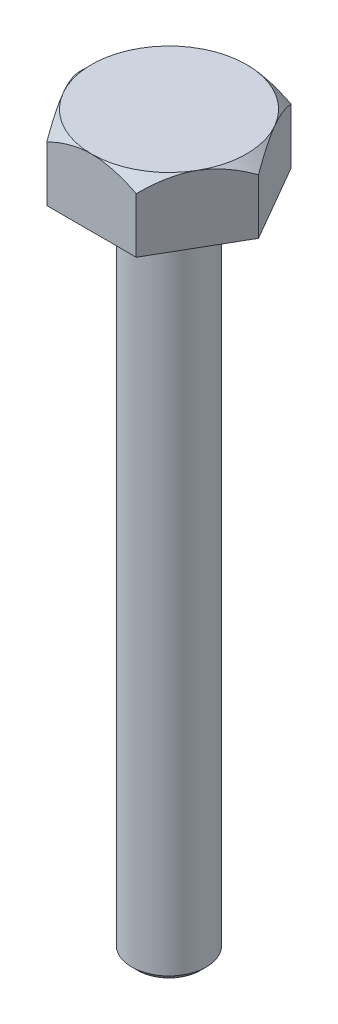
ISO-10303-21;
HEADER;
FILE_DESCRIPTION(('STEP AP214'),'2;1');
FILE_NAME('part.step','',(''),(''),'','','');
FILE_SCHEMA(('AUTOMOTIVE_DESIGN { 1 0 10303 214 1 1 1 1 }'));
ENDSEC;
DATA;
#1=APPLICATION_CONTEXT('core data for automotive mechanical design processes');
#2=APPLICATION_PROTOCOL_DEFINITION('international standard','automotive_design',2000,#1);
#3=PRODUCT_CONTEXT('',#1,'mechanical');
#4=PRODUCT('Part','Part','',(#3));
#5=PRODUCT_RELATED_PRODUCT_CATEGORY('part','',(#4));
#6=PRODUCT_DEFINITION_FORMATION('','',#4);
#7=PRODUCT_DEFINITION_CONTEXT('part definition',#1,'design');
#8=PRODUCT_DEFINITION('design','',#6,#7);
#9=PRODUCT_DEFINITION_SHAPE('','',#8);
#10=(LENGTH_UNIT() NAMED_UNIT(*) SI_UNIT(.MILLI.,.METRE.));
#11=(NAMED_UNIT(*) PLANE_ANGLE_UNIT() SI_UNIT($,.RADIAN.));
#12=(NAMED_UNIT(*) SI_UNIT($,.STERADIAN.) SOLID_ANGLE_UNIT());
#13=UNCERTAINTY_MEASURE_WITH_UNIT(LENGTH_MEASURE(1.E-05),#10,'distance_accuracy_value','');
#14=(GEOMETRIC_REPRESENTATION_CONTEXT(3) GLOBAL_UNCERTAINTY_ASSIGNED_CONTEXT((#13)) GLOBAL_UNIT_ASSIGNED_CONTEXT((#10,
#11,#12)) REPRESENTATION_CONTEXT('',''));
#15=CARTESIAN_POINT('',(0.,0.,0.));
#16=DIRECTION('',(0.,0.,1.));
#17=DIRECTION('',(1.,0.,0.));
#18=AXIS2_PLACEMENT_3D('',#15,#16,#17);
#19=CARTESIAN_POINT('',(-30.0222139978605,45.,52.));
#20=DIRECTION('',(0.,0.,-1.));
#21=DIRECTION('',(-1.,0.,0.));
#22=AXIS2_PLACEMENT_3D('',#19,#20,#21);
#23=PLANE('',#22);
#24=CARTESIAN_POINT('',(-104.974603519539,-20.1480575344053,52.));
#25=CARTESIAN_POINT('',(-103.444442169708,-18.7769494356472,52.));
#26=CARTESIAN_POINT('',(-101.911384838102,-17.4090635637915,52.));
#27=CARTESIAN_POINT('',(-98.8386625300546,-14.680700729552,52.));
#28=CARTESIAN_POINT('',(-97.2989974806682,-13.3202238493363,52.));
#29=CARTESIAN_POINT('',(-94.2117655194995,-10.6072235850642,52.));
#30=CARTESIAN_POINT('',(-92.664196154111,-9.25470299139133,52.));
#31=CARTESIAN_POINT('',(-89.5606976427889,-6.55929062983141,52.));
#32=CARTESIAN_POINT('',(-88.0047685189832,-5.2163988364791,52.));
#33=CARTESIAN_POINT('',(-84.8665982537161,-2.52727361111867,52.));
#34=CARTESIAN_POINT('',(-83.2842542569196,-1.18116012717798,52.));
#35=CARTESIAN_POINT('',(-80.1084838043138,1.49794750629656,52.));
#36=CARTESIAN_POINT('',(-78.5150573248629,2.83094162782893,52.));
#37=CARTESIAN_POINT('',(-75.3157667376626,5.48135702448698,52.));
#38=CARTESIAN_POINT('',(-73.7099048716653,6.79878100306021,52.));
#39=CARTESIAN_POINT('',(-70.4835124655795,9.4155570233478,52.));
#40=CARTESIAN_POINT('',(-68.8629819723785,10.7149091227943,52.));
#41=CARTESIAN_POINT('',(-65.7252946964395,13.1968820674329,52.));
#42=CARTESIAN_POINT('',(-64.2093494345498,14.3810328857299,52.));
#43=CARTESIAN_POINT('',(-61.1606138406127,16.7275072656802,52.));
#44=CARTESIAN_POINT('',(-59.6278234019294,17.8898306890322,52.));
#45=CARTESIAN_POINT('',(-56.5419574813941,20.1889777107931,52.));
#46=CARTESIAN_POINT('',(-54.9888717926023,21.3257876303724,52.));
#47=CARTESIAN_POINT('',(-51.8600616034661,23.5678926917397,52.));
#48=CARTESIAN_POINT('',(-50.2843374479378,24.6731883127718,52.));
#49=CARTESIAN_POINT('',(-47.9027588961038,26.3010577204605,52.));
#50=CARTESIAN_POINT('',(-47.1067786209454,26.8380990869268,52.));
#51=CARTESIAN_POINT('',(-45.5077429876137,27.9015346461807,52.));
#52=CARTESIAN_POINT('',(-44.7046877300736,28.4279289900598,52.));
#53=CARTESIAN_POINT('',(-43.09085839563,29.4689559851113,52.));
#54=CARTESIAN_POINT('',(-42.2800834844557,29.9835873441311,52.));
#55=CARTESIAN_POINT('',(-40.6503308676235,30.9996707599405,52.));
#56=CARTESIAN_POINT('',(-39.8313533365432,31.5011230964014,52.));
#57=CARTESIAN_POINT('',(-38.1852760607041,32.4888985857804,52.));
#58=CARTESIAN_POINT('',(-37.3581839506433,32.975234444567,52.));
#59=CARTESIAN_POINT('',(-35.6945351895526,33.9314936100802,52.));
#60=CARTESIAN_POINT('',(-34.8579784034972,34.4014166822659,52.));
#61=CARTESIAN_POINT('',(-33.1749408969925,35.3227686623054,52.));
#62=CARTESIAN_POINT('',(-32.3284621837012,35.7742012304012,52.));
#63=CARTESIAN_POINT('',(-30.6248353182834,36.6564043219331,52.));
#64=CARTESIAN_POINT('',(-29.7676877068093,37.0871758870515,52.));
#65=CARTESIAN_POINT('',(-28.1014002469777,37.8967384425179,52.));
#66=CARTESIAN_POINT('',(-27.2930086854749,38.2770672919812,52.));
#67=CARTESIAN_POINT('',(-25.6660607005647,39.0153364246869,52.));
#68=CARTESIAN_POINT('',(-24.8475044775925,39.3732771485594,52.));
#69=CARTESIAN_POINT('',(-23.1998803156875,40.0642892826952,52.));
#70=CARTESIAN_POINT('',(-22.3708117857534,40.3973592874115,52.));
#71=CARTESIAN_POINT('',(-20.702073505453,41.0358896387952,52.));
#72=CARTESIAN_POINT('',(-19.862403698907,41.3413498390793,52.));
#73=CARTESIAN_POINT('',(-18.1762063413501,41.9205092993988,52.));
#74=CARTESIAN_POINT('',(-17.3297241511565,42.1943402003845,52.));
#75=CARTESIAN_POINT('',(-15.626734785493,42.7087845664855,52.));
#76=CARTESIAN_POINT('',(-14.7702281113905,42.949399685228,52.));
#77=CARTESIAN_POINT('',(-13.0478359049288,43.3944593584753,52.));
#78=CARTESIAN_POINT('',(-12.1819504308002,43.5989041374158,52.));
#79=CARTESIAN_POINT('',(-10.4418517197723,43.9687867466574,52.));
#80=CARTESIAN_POINT('',(-9.56763847282889,44.134224529906,52.));
#81=CARTESIAN_POINT('',(-7.79708737906465,44.4260605485028,52.));
#82=CARTESIAN_POINT('',(-6.9006289245866,44.5517311226506,52.));
#83=CARTESIAN_POINT('',(-5.10250864919229,44.7578905629406,52.));
#84=CARTESIAN_POINT('',(-4.20084684342538,44.8383795605602,52.));
#85=CARTESIAN_POINT('',(-2.39467100795442,44.9526915724833,52.));
#86=CARTESIAN_POINT('',(-1.49015736317976,44.9865206354127,52.));
#87=CARTESIAN_POINT('',(0.319405672869893,45.006889864112,52.));
#88=CARTESIAN_POINT('',(1.22445506460228,44.9934299894499,52.));
#89=CARTESIAN_POINT('',(3.03386911749646,44.919427081205,52.));
#90=CARTESIAN_POINT('',(3.93823110670625,44.8588190475472,52.));
#91=CARTESIAN_POINT('',(5.74266334205835,44.6915772321508,52.));
#92=CARTESIAN_POINT('',(6.64273359815255,44.5849435571916,52.));
#93=CARTESIAN_POINT('',(8.4367191402026,44.3275220036307,52.));
#94=CARTESIAN_POINT('',(9.3306329712175,44.1767240310471,52.));
#95=CARTESIAN_POINT('',(11.1104092248204,43.8334830356432,52.));
#96=CARTESIAN_POINT('',(11.9962713736148,43.6410386021344,52.));
#97=CARTESIAN_POINT('',(13.9673809097387,43.1672161224463,52.));
#98=CARTESIAN_POINT('',(15.050162325768,42.8755698359679,52.));
#99=CARTESIAN_POINT('',(17.199882392269,42.2388692101925,52.));
#100=CARTESIAN_POINT('',(18.2668196987303,41.8938103681036,52.));
#101=CARTESIAN_POINT('',(20.3844311305142,41.1561144157292,52.));
#102=CARTESIAN_POINT('',(21.435099820739,40.7634617760078,52.));
#103=CARTESIAN_POINT('',(23.5197432427476,39.9363267728805,52.));
#104=CARTESIAN_POINT('',(24.5537182535443,39.5018451094386,52.));
#105=CARTESIAN_POINT('',(26.617528684912,38.5908799093831,52.));
#106=CARTESIAN_POINT('',(27.6471714147959,38.1139613893689,52.));
#107=CARTESIAN_POINT('',(29.6905952704967,37.127377922496,52.));
#108=CARTESIAN_POINT('',(30.7043763240441,36.6177128264905,52.));
#109=CARTESIAN_POINT('',(32.7167190987185,35.5699916340616,52.));
#110=CARTESIAN_POINT('',(33.7152855879172,35.0319446782918,52.));
#111=CARTESIAN_POINT('',(35.2027091269047,34.2062038320033,52.));
#112=CARTESIAN_POINT('',(35.6967798168579,33.927844828386,52.));
#113=CARTESIAN_POINT('',(36.6815952247146,33.3652920044684,52.));
#114=CARTESIAN_POINT('',(37.1723399145891,33.0810981350774,52.));
#115=CARTESIAN_POINT('',(38.4627450247686,32.3241817303639,52.));
#116=CARTESIAN_POINT('',(39.2597166191444,31.8468695967498,52.));
#117=CARTESIAN_POINT('',(40.8456504803188,30.8791046473685,52.));
#118=CARTESIAN_POINT('',(41.634612523387,30.3886514659184,52.));
#119=CARTESIAN_POINT('',(43.9904571033975,28.8995073949854,52.));
#120=CARTESIAN_POINT('',(45.5461685713643,27.883108504139,52.));
#121=CARTESIAN_POINT('',(48.6324575998831,25.8114617071009,52.));
#122=CARTESIAN_POINT('',(50.1630226887238,24.7561953178764,52.));
#123=CARTESIAN_POINT('',(53.201750110714,22.6140796743748,52.));
#124=CARTESIAN_POINT('',(54.7099133781582,21.5272317428642,52.));
#125=CARTESIAN_POINT('',(57.710912846122,19.3243364554514,52.));
#126=CARTESIAN_POINT('',(59.2036974407832,18.2082189541388,52.));
#127=CARTESIAN_POINT('',(62.1724441153612,15.9538389324413,52.));
#128=CARTESIAN_POINT('',(63.6484060467436,14.815576216767,52.));
#129=CARTESIAN_POINT('',(66.5853088929478,12.5206289542413,52.));
#130=CARTESIAN_POINT('',(68.0462535581434,11.3639492002705,52.));
#131=CARTESIAN_POINT('',(70.9553551542158,9.0346475086844,52.));
#132=CARTESIAN_POINT('',(72.4035121356618,7.86202563415925,52.));
#133=CARTESIAN_POINT('',(75.1757977039992,5.59532448057323,52.));
#134=CARTESIAN_POINT('',(76.5007688916879,4.50227464071074,52.));
#135=CARTESIAN_POINT('',(79.1422374587787,2.3059909642823,52.));
#136=CARTESIAN_POINT('',(80.4587348436884,1.20275713433677,52.));
#137=CARTESIAN_POINT('',(83.0842587401692,-1.01274333093366,52.));
#138=CARTESIAN_POINT('',(84.3932847278744,-2.12501058671541,52.));
#139=CARTESIAN_POINT('',(87.0045660739479,-4.35746560380634,52.));
#140=CARTESIAN_POINT('',(88.3068214204755,-5.47765337895888,52.));
#141=CARTESIAN_POINT('',(90.8973931655344,-7.71826962519173,52.));
#142=CARTESIAN_POINT('',(92.185746238517,-8.83865571159717,52.));
#143=CARTESIAN_POINT('',(94.7570301747009,-11.0856338234656,52.));
#144=CARTESIAN_POINT('',(96.0399610313417,-12.2122258564337,52.));
#145=CARTESIAN_POINT('',(98.6007446717763,-14.4708145356289,52.));
#146=CARTESIAN_POINT('',(99.8785981218244,-15.6028104267575,52.));
#147=CARTESIAN_POINT('',(102.42983830778,-17.8718111259995,52.));
#148=CARTESIAN_POINT('',(103.703225068163,-19.0088159065893,52.));
#149=CARTESIAN_POINT('',(104.974603519539,-20.1480575344052,52.));
#150=B_SPLINE_CURVE_WITH_KNOTS('',3,(#24,#25,#26,#27,#28,#29,#30,#31,#32,#33,#34,#35,#36,#37,
#38,#39,#40,#41,#42,#43,#44,#45,#46,#47,#48,#49,#50,#51,#52,#53,#54,#55,#56,#57,#58,#59,#60,#61,
#62,#63,#64,#65,#66,#67,#68,#69,#70,#71,#72,#73,#74,#75,#76,#77,#78,#79,#80,#81,#82,#83,#84,#85,
#86,#87,#88,#89,#90,#91,#92,#93,#94,#95,#96,#97,#98,#99,#100,#101,#102,#103,#104,#105,#106,#107,
#108,#109,#110,#111,#112,#113,#114,#115,#116,#117,#118,#119,#120,#121,#122,#123,#124,#125,#126,
#127,#128,#129,#130,#131,#132,#133,#134,#135,#136,#137,#138,#139,#140,#141,#142,#143,#144,#145,
#146,#147,#148,#149),.UNSPECIFIED.,.F.,.F.,(4,2,2,2,2,2,2,2,2,2,2,2,2,2,2,2,2,2,2,2,2,2,2,2,2,2,
2,2,2,2,2,2,2,2,2,2,2,2,2,2,2,2,2,2,2,2,2,2,2,2,2,2,2,2,2,2,2,2,2,2,2,2,4),(0.,6.16376855195753,
12.3276053234916,18.493488395418,24.6593551544522,30.8916696404896,37.1239974256607,
43.3552267046366,49.5864360728412,55.3571233374888,61.1278471536516,66.9015943485739,
72.6752536941409,75.5558064266588,78.4363182526549,81.3171449940328,84.1979105520807,
87.0761853944353,89.9545013508952,92.8322447563134,95.7098429194175,98.3897109444312,
101.069526209232,103.74949280703,106.429473612808,109.09786454091,111.766122576876,
114.434364055812,117.102608753327,119.817178750423,122.531740848134,125.245951018343,
127.960163509202,130.678124552666,133.396079290505,136.114655716595,138.833324243306,
142.19585187024,145.558663119932,148.922574594002,152.286429786384,155.689963480925,
159.093512678226,162.495972343473,164.197205953724,165.898453882901,168.685217983057,
171.472059712695,177.046194286842,182.623014702026,188.199601872464,193.791062080716,
199.382571620079,204.972649057908,210.562704379728,215.715585071901,220.868462414519,
226.021696724868,231.174940044188,236.297033600975,241.419133353498,246.540537187855,
251.661912915344),.UNSPECIFIED.);
#151=CARTESIAN_POINT('',(-30.0222139978605,36.9555720042789,52.));
#152=VERTEX_POINT('',#151);
#153=CARTESIAN_POINT('',(0.,45.,52.));
#154=VERTEX_POINT('',#153);
#155=EDGE_CURVE('E222',#152,#154,#150,.T.);
#156=ORIENTED_EDGE('',*,*,#155,.F.);
#157=DIRECTION('',(0.,-1.,0.));
#158=VECTOR('',#157,1.);
#159=CARTESIAN_POINT('',(-30.0222139978605,45.,52.));
#160=LINE('',#159,#158);
#161=CARTESIAN_POINT('',(-30.0222139978605,0.,52.));
#162=VERTEX_POINT('',#161);
#163=EDGE_CURVE('E221',#152,#162,#160,.T.);
#164=ORIENTED_EDGE('',*,*,#163,.T.);
#165=DIRECTION('',(1.,0.,0.));
#166=VECTOR('',#165,1.);
#167=CARTESIAN_POINT('',(-30.0222139978605,0.,52.));
#168=LINE('',#167,#166);
#169=CARTESIAN_POINT('',(30.0222139978605,0.,52.));
#170=VERTEX_POINT('',#169);
#171=EDGE_CURVE('E228',#162,#170,#168,.T.);
#172=ORIENTED_EDGE('',*,*,#171,.T.);
#173=DIRECTION('',(0.,-1.,0.));
#174=VECTOR('',#173,1.);
#175=CARTESIAN_POINT('',(30.0222139978605,45.,52.));
#176=LINE('',#175,#174);
#177=CARTESIAN_POINT('',(30.0222139978605,36.9555720042789,52.));
#178=VERTEX_POINT('',#177);
#179=EDGE_CURVE('E247',#178,#170,#176,.T.);
#180=ORIENTED_EDGE('',*,*,#179,.F.);
#181=EDGE_CURVE('E116',#154,#178,#150,.T.);
#182=ORIENTED_EDGE('',*,*,#181,.F.);
#183=EDGE_LOOP('',(#156,#164,#172,#180,#182));
#184=FACE_BOUND('',#183,.T.);
#185=ADVANCED_FACE('F45',(#184),#23,.F.);
#186=CARTESIAN_POINT('',(30.0222139978605,45.,52.));
#187=DIRECTION('',(-0.866025403784438,0.,-0.5));
#188=DIRECTION('',(-0.5,0.,0.866025403784439));
#189=AXIS2_PLACEMENT_3D('',#186,#187,#188);
#190=PLANE('',#189);
#191=CARTESIAN_POINT('',(30.0220985278067,36.955456533892,52.0002));
#192=CARTESIAN_POINT('',(30.280176534641,37.2135309803307,51.5531957798468));
#193=CARTESIAN_POINT('',(30.5392485388566,37.4676183415671,51.1044699057268));
#194=CARTESIAN_POINT('',(31.0594616022098,37.9672410148882,50.2034344492379));
#195=CARTESIAN_POINT('',(31.3206027677406,38.212775883668,49.7511246825909));
#196=CARTESIAN_POINT('',(32.107464297322,38.9358777611029,48.3882405348345));
#197=CARTESIAN_POINT('',(32.6363738806571,39.3996919544938,47.4721422638881));
#198=CARTESIAN_POINT('',(33.7060127767282,40.2877490866143,45.619473350141));
#199=CARTESIAN_POINT('',(34.2467924232445,40.7117502689875,44.6828155266756));
#200=CARTESIAN_POINT('',(35.3372385336309,41.5110185100584,42.7941074605706));
#201=CARTESIAN_POINT('',(35.8869036244094,41.8862930191751,41.8420595961952));
#202=CARTESIAN_POINT('',(36.9862330817044,42.5761964413529,39.9379651219031));
#203=CARTESIAN_POINT('',(37.5357617449106,42.8916856332666,38.9861535570145));
#204=CARTESIAN_POINT('',(38.6426137983935,43.462897464706,37.0690295639203));
#205=CARTESIAN_POINT('',(39.1999375700364,43.7186171691656,36.1037164751688));
#206=CARTESIAN_POINT('',(40.3198432183338,44.1637824175714,34.1639829926344));
#207=CARTESIAN_POINT('',(40.8824096700677,44.3533822155406,33.1895893155975));
#208=CARTESIAN_POINT('',(42.0123359693659,44.6621218387154,31.2324995564048));
#209=CARTESIAN_POINT('',(42.5796950878927,44.7812721913383,30.2498047369788));
#210=CARTESIAN_POINT('',(43.5552992194105,44.9223807751639,28.5600088131159));
#211=CARTESIAN_POINT('',(43.9629124532236,44.9623420710016,27.8540019823142));
#212=CARTESIAN_POINT('',(44.7786213959163,45.0038958786488,26.4411526493822));
#213=CARTESIAN_POINT('',(45.1867170795089,45.0054903193645,25.7343101910502));
#214=CARTESIAN_POINT('',(46.0026361970847,44.9702724935875,24.3210968245421));
#215=CARTESIAN_POINT('',(46.4104594797881,44.9334463746507,23.6147261783904));
#216=CARTESIAN_POINT('',(47.2248121036791,44.8219352098245,22.204226058534));
#217=CARTESIAN_POINT('',(47.6313414225626,44.747249514863,21.5000966234615));
#218=CARTESIAN_POINT('',(48.4427192287144,44.5610301112822,20.0947490390728));
#219=CARTESIAN_POINT('',(48.8475654352428,44.4494568192073,19.3935348401141));
#220=CARTESIAN_POINT('',(49.6544259013264,44.191061053402,17.9960115182386));
#221=CARTESIAN_POINT('',(50.0564401456341,44.044238390037,17.2997024217312));
#222=CARTESIAN_POINT('',(50.8569901438334,43.7172974585385,15.9131091508509));
#223=CARTESIAN_POINT('',(51.255526460246,43.537184683344,15.222824002163));
#224=CARTESIAN_POINT('',(52.0487663374305,43.1458008444998,13.8488922322897));
#225=CARTESIAN_POINT('',(52.4434695874179,42.9345272764499,13.165246149399));
#226=CARTESIAN_POINT('',(53.4596132305348,42.3503586126167,11.4052337317323));
#227=CARTESIAN_POINT('',(54.0779115662168,41.9554756092821,10.3343096000959));
#228=CARTESIAN_POINT('',(55.3033387530697,41.1021232134822,8.21180745149049));
#229=CARTESIAN_POINT('',(55.9104672666288,40.6436519026025,7.16023001928237));
#230=CARTESIAN_POINT('',(57.1117585467271,39.6733005330436,5.07953248746263));
#231=CARTESIAN_POINT('',(57.7059553438547,39.1615884431307,4.05035344514291));
#232=CARTESIAN_POINT('',(58.589037605449,38.3591005271834,2.5208101007988));
#233=CARTESIAN_POINT('',(58.8819529950742,38.0858616283834,2.01346576364905));
#234=CARTESIAN_POINT('',(59.4651752455835,37.5285665756802,1.00329519366237));
#235=CARTESIAN_POINT('',(59.7554822933588,37.2445112045562,0.500468637120165));
#236=CARTESIAN_POINT('',(60.0445434657749,36.955456533892,-0.000200000000003977));
#237=B_SPLINE_CURVE_WITH_KNOTS('',3,(#191,#192,#193,#194,#195,#196,#197,#198,#199,#200,#201,
#202,#203,#204,#205,#206,#207,#208,#209,#210,#211,#212,#213,#214,#215,#216,#217,#218,#219,#220,
#221,#222,#223,#224,#225,#226,#227,#228,#229,#230,#231,#232,#233,#234,#235,#236),.UNSPECIFIED.,
.F.,.F.,(4,2,2,2,2,2,2,2,2,2,2,2,2,2,2,2,2,2,2,2,2,2,4),(0.,1.73120255917828,3.46249471937643,
6.92674897903961,10.4108367985433,13.8943912642056,17.3232079778035,20.7521930329862,
24.1731240857042,27.5935438118124,30.041323321998,32.4889797690039,34.9375190179709,
37.3861002466024,39.8373175810715,42.2885481029052,44.7393745269956,47.1903980320222,
51.0825946301762,54.9749086787068,58.8552952790952,60.7944610079083,62.733486666627),.UNSPECIFIED.);
#238=CARTESIAN_POINT('',(45.0333209967908,45.,26.));
#239=VERTEX_POINT('',#238);
#240=EDGE_CURVE('E111',#178,#239,#237,.T.);
#241=ORIENTED_EDGE('',*,*,#240,.F.);
#242=ORIENTED_EDGE('',*,*,#179,.T.);
#243=DIRECTION('',(0.5,0.,-0.866025403784438));
#244=VECTOR('',#243,1.);
#245=CARTESIAN_POINT('',(30.0222139978605,0.,52.));
#246=LINE('',#245,#244);
#247=CARTESIAN_POINT('',(60.0444279957211,0.,0.));
#248=VERTEX_POINT('',#247);
#249=EDGE_CURVE('E257',#170,#248,#246,.T.);
#250=ORIENTED_EDGE('',*,*,#249,.T.);
#251=DIRECTION('',(0.,-1.,0.));
#252=VECTOR('',#251,1.);
#253=CARTESIAN_POINT('',(60.0444279957211,45.,0.));
#254=LINE('',#253,#252);
#255=CARTESIAN_POINT('',(60.0444279957211,36.9555720042789,0.));
#256=VERTEX_POINT('',#255);
#257=EDGE_CURVE('E141',#256,#248,#254,.T.);
#258=ORIENTED_EDGE('',*,*,#257,.F.);
#259=EDGE_CURVE('E124',#239,#256,#237,.T.);
#260=ORIENTED_EDGE('',*,*,#259,.F.);
#261=EDGE_LOOP('',(#241,#242,#250,#258,#260));
#262=FACE_BOUND('',#261,.T.);
#263=ADVANCED_FACE('F143',(#262),#190,.F.);
#264=CARTESIAN_POINT('',(60.0444279957211,45.,0.));
#265=DIRECTION('',(-0.866025403784439,0.,0.5));
#266=DIRECTION('',(0.5,0.,0.866025403784439));
#267=AXIS2_PLACEMENT_3D('',#264,#265,#266);
#268=PLANE('',#267);
#269=CARTESIAN_POINT('',(60.0445434657749,36.955456533892,0.000199999999997052));
#270=CARTESIAN_POINT('',(59.7864654589406,37.2135309803307,-0.446804220153167));
#271=CARTESIAN_POINT('',(59.527393454725,37.4676183415671,-0.895530094273238));
#272=CARTESIAN_POINT('',(59.0071803913718,37.9672410148882,-1.7965655507621));
#273=CARTESIAN_POINT('',(58.746039225841,38.212775883668,-2.24887531740914));
#274=CARTESIAN_POINT('',(57.9591776962596,38.9358777611029,-3.61175946516546));
#275=CARTESIAN_POINT('',(57.4302681129245,39.3996919544938,-4.52785773611194));
#276=CARTESIAN_POINT('',(56.3606292168534,40.2877490866143,-6.38052664985905));
#277=CARTESIAN_POINT('',(55.8198495703371,40.7117502689875,-7.31718447332443));
#278=CARTESIAN_POINT('',(54.7294034599507,41.5110185100584,-9.20589253942941));
#279=CARTESIAN_POINT('',(54.1797383691722,41.8862930191751,-10.1579404038048));
#280=CARTESIAN_POINT('',(53.0804089118772,42.5761964413529,-12.0620348780969));
#281=CARTESIAN_POINT('',(52.530880248671,42.8916856332666,-13.0138464429855));
#282=CARTESIAN_POINT('',(51.4240281951881,43.462897464706,-14.9309704360797));
#283=CARTESIAN_POINT('',(50.8667044235452,43.7186171691656,-15.8962835248312));
#284=CARTESIAN_POINT('',(49.7467987752478,44.1637824175714,-17.8360170073656));
#285=CARTESIAN_POINT('',(49.1842323235139,44.3533822155406,-18.8104106844025));
#286=CARTESIAN_POINT('',(48.0543060242157,44.6621218387154,-20.7675004435952));
#287=CARTESIAN_POINT('',(47.4869469056889,44.7812721913382,-21.7501952630212));
#288=CARTESIAN_POINT('',(46.5113427741711,44.9223807751638,-23.4399911868841));
#289=CARTESIAN_POINT('',(46.103729540358,44.9623420710016,-24.1459980176858));
#290=CARTESIAN_POINT('',(45.2880205976653,45.0038958786488,-25.5588473506178));
#291=CARTESIAN_POINT('',(44.8799249140727,45.0054903193645,-26.2656898089498));
#292=CARTESIAN_POINT('',(44.0640057964969,44.9702724935875,-27.6789031754579));
#293=CARTESIAN_POINT('',(43.6561825137935,44.9334463746507,-28.3852738216097));
#294=CARTESIAN_POINT('',(42.8418298899025,44.8219352098245,-29.795773941466));
#295=CARTESIAN_POINT('',(42.435300571019,44.747249514863,-30.4999033765385));
#296=CARTESIAN_POINT('',(41.6239227648672,44.5610301112822,-31.9052509609272));
#297=CARTESIAN_POINT('',(41.2190765583388,44.4494568192073,-32.606465159886));
#298=CARTESIAN_POINT('',(40.4122160922552,44.191061053402,-34.0039884817614));
#299=CARTESIAN_POINT('',(40.0102018479474,44.044238390037,-34.7002975782688));
#300=CARTESIAN_POINT('',(39.2096518497482,43.7172974585385,-36.0868908491491));
#301=CARTESIAN_POINT('',(38.8111155333356,43.537184683344,-36.777175997837));
#302=CARTESIAN_POINT('',(38.0178756561511,43.1458008444998,-38.1511077677104));
#303=CARTESIAN_POINT('',(37.6231724061637,42.9345272764499,-38.834753850601));
#304=CARTESIAN_POINT('',(36.6070287630468,42.3503586126167,-40.5947662682677));
#305=CARTESIAN_POINT('',(35.9887304273648,41.9554756092821,-41.6656903999042));
#306=CARTESIAN_POINT('',(34.7633032405119,41.1021232134821,-43.7881925485095));
#307=CARTESIAN_POINT('',(34.1561747269528,40.6436519026025,-44.8397699807176));
#308=CARTESIAN_POINT('',(32.9548834468545,39.6733005330436,-46.9204675125374));
#309=CARTESIAN_POINT('',(32.3606866497269,39.1615884431307,-47.9496465548571));
#310=CARTESIAN_POINT('',(31.4776043881327,38.3591005271834,-49.4791898992012));
#311=CARTESIAN_POINT('',(31.1846889985074,38.0858616283834,-49.9865342363509));
#312=CARTESIAN_POINT('',(30.6014667479982,37.5285665756802,-50.9967048063376));
#313=CARTESIAN_POINT('',(30.3111597002228,37.2445112045562,-51.4995313628798));
#314=CARTESIAN_POINT('',(30.0220985278067,36.955456533892,-52.0002));
#315=B_SPLINE_CURVE_WITH_KNOTS('',3,(#269,#270,#271,#272,#273,#274,#275,#276,#277,#278,#279,
#280,#281,#282,#283,#284,#285,#286,#287,#288,#289,#290,#291,#292,#293,#294,#295,#296,#297,#298,
#299,#300,#301,#302,#303,#304,#305,#306,#307,#308,#309,#310,#311,#312,#313,#314),.UNSPECIFIED.,
.F.,.F.,(4,2,2,2,2,2,2,2,2,2,2,2,2,2,2,2,2,2,2,2,2,2,4),(0.,1.73120255917828,3.46249471937644,
6.92674897903963,10.4108367985433,13.8943912642057,17.3232079778035,20.7521930329862,
24.1731240857042,27.5935438118124,30.0413233219981,32.4889797690039,34.937519017971,
37.3861002466024,39.8373175810715,42.2885481029052,44.7393745269956,47.1903980320223,
51.0825946301762,54.9749086787068,58.8552952790952,60.7944610079083,62.733486666627),.UNSPECIFIED.);
#316=CARTESIAN_POINT('',(45.0333209967908,45.,-26.));
#317=VERTEX_POINT('',#316);
#318=EDGE_CURVE('E129',#256,#317,#315,.T.);
#319=ORIENTED_EDGE('',*,*,#318,.F.);
#320=ORIENTED_EDGE('',*,*,#257,.T.);
#321=DIRECTION('',(-0.5,0.,-0.866025403784439));
#322=VECTOR('',#321,1.);
#323=CARTESIAN_POINT('',(60.0444279957211,0.,0.));
#324=LINE('',#323,#322);
#325=CARTESIAN_POINT('',(30.0222139978605,0.,-52.));
#326=VERTEX_POINT('',#325);
#327=EDGE_CURVE('E261',#248,#326,#324,.T.);
#328=ORIENTED_EDGE('',*,*,#327,.T.);
#329=DIRECTION('',(0.,-1.,0.));
#330=VECTOR('',#329,1.);
#331=CARTESIAN_POINT('',(30.0222139978605,45.,-52.));
#332=LINE('',#331,#330);
#333=CARTESIAN_POINT('',(30.0222139978605,36.9555720042789,-52.));
#334=VERTEX_POINT('',#333);
#335=EDGE_CURVE('E241',#334,#326,#332,.T.);
#336=ORIENTED_EDGE('',*,*,#335,.F.);
#337=EDGE_CURVE('E145',#317,#334,#315,.T.);
#338=ORIENTED_EDGE('',*,*,#337,.F.);
#339=EDGE_LOOP('',(#319,#320,#328,#336,#338));
#340=FACE_BOUND('',#339,.T.);
#341=ADVANCED_FACE('F206',(#340),#268,.F.);
#342=CARTESIAN_POINT('',(30.0222139978605,45.,-52.));
#343=DIRECTION('',(0.,0.,1.));
#344=DIRECTION('',(1.,0.,0.));
#345=AXIS2_PLACEMENT_3D('',#342,#343,#344);
#346=PLANE('',#345);
#347=CARTESIAN_POINT('',(104.974603519539,-20.1480575344053,-52.));
#348=CARTESIAN_POINT('',(103.444442169708,-18.7769494356472,-52.));
#349=CARTESIAN_POINT('',(101.911384838102,-17.4090635637915,-52.));
#350=CARTESIAN_POINT('',(98.8386625300547,-14.680700729552,-52.));
#351=CARTESIAN_POINT('',(97.2989974806683,-13.3202238493364,-52.));
#352=CARTESIAN_POINT('',(94.2117655194995,-10.6072235850642,-52.));
#353=CARTESIAN_POINT('',(92.6641961541111,-9.25470299139135,-52.));
#354=CARTESIAN_POINT('',(89.5606976427889,-6.55929062983143,-52.));
#355=CARTESIAN_POINT('',(88.0047685189833,-5.21639883647913,-52.));
#356=CARTESIAN_POINT('',(84.8665982537161,-2.52727361111871,-52.));
#357=CARTESIAN_POINT('',(83.2842542569196,-1.181160127178,-52.));
#358=CARTESIAN_POINT('',(80.1084838043138,1.49794750629655,-52.));
#359=CARTESIAN_POINT('',(78.5150573248629,2.83094162782891,-52.));
#360=CARTESIAN_POINT('',(75.3157667376626,5.48135702448695,-52.));
#361=CARTESIAN_POINT('',(73.7099048716654,6.79878100306017,-52.));
#362=CARTESIAN_POINT('',(70.4835124655795,9.41555702334776,-52.));
#363=CARTESIAN_POINT('',(68.8629819723785,10.7149091227943,-52.));
#364=CARTESIAN_POINT('',(65.7252946964395,13.1968820674329,-52.));
#365=CARTESIAN_POINT('',(64.2093494345498,14.3810328857299,-52.));
#366=CARTESIAN_POINT('',(61.1606138406127,16.7275072656802,-52.));
#367=CARTESIAN_POINT('',(59.6278234019294,17.8898306890322,-52.));
#368=CARTESIAN_POINT('',(56.5419574813941,20.1889777107931,-52.));
#369=CARTESIAN_POINT('',(54.9888717926024,21.3257876303723,-52.));
#370=CARTESIAN_POINT('',(51.8600616034662,23.5678926917397,-52.));
#371=CARTESIAN_POINT('',(50.2843374479378,24.6731883127717,-52.));
#372=CARTESIAN_POINT('',(47.9027588961038,26.3010577204604,-52.));
#373=CARTESIAN_POINT('',(47.1067786209455,26.8380990869267,-52.));
#374=CARTESIAN_POINT('',(45.5077429876137,27.9015346461807,-52.));
#375=CARTESIAN_POINT('',(44.7046877300736,28.4279289900597,-52.));
#376=CARTESIAN_POINT('',(43.09085839563,29.4689559851113,-52.));
#377=CARTESIAN_POINT('',(42.2800834844558,29.9835873441311,-52.));
#378=CARTESIAN_POINT('',(40.6503308676236,30.9996707599404,-52.));
#379=CARTESIAN_POINT('',(39.8313533365432,31.5011230964014,-52.));
#380=CARTESIAN_POINT('',(38.1852760607041,32.4888985857804,-52.));
#381=CARTESIAN_POINT('',(37.3581839506433,32.975234444567,-52.));
#382=CARTESIAN_POINT('',(35.6945351895526,33.9314936100802,-52.));
#383=CARTESIAN_POINT('',(34.8579784034973,34.4014166822659,-52.));
#384=CARTESIAN_POINT('',(33.1749408969925,35.3227686623054,-52.));
#385=CARTESIAN_POINT('',(32.3284621837013,35.7742012304011,-52.));
#386=CARTESIAN_POINT('',(30.6248353182834,36.6564043219331,-52.));
#387=CARTESIAN_POINT('',(29.7676877068093,37.0871758870515,-52.));
#388=CARTESIAN_POINT('',(28.1014002469778,37.8967384425179,-52.));
#389=CARTESIAN_POINT('',(27.2930086854749,38.2770672919812,-52.));
#390=CARTESIAN_POINT('',(25.6660607005647,39.0153364246868,-52.));
#391=CARTESIAN_POINT('',(24.8475044775926,39.3732771485593,-52.));
#392=CARTESIAN_POINT('',(23.1998803156876,40.0642892826952,-52.));
#393=CARTESIAN_POINT('',(22.3708117857535,40.3973592874115,-52.));
#394=CARTESIAN_POINT('',(20.7020735054531,41.0358896387952,-52.));
#395=CARTESIAN_POINT('',(19.8624036989071,41.3413498390792,-52.));
#396=CARTESIAN_POINT('',(18.1762063413502,41.9205092993988,-52.));
#397=CARTESIAN_POINT('',(17.3297241511565,42.1943402003845,-52.));
#398=CARTESIAN_POINT('',(15.626734785493,42.7087845664855,-52.));
#399=CARTESIAN_POINT('',(14.7702281113905,42.949399685228,-52.));
#400=CARTESIAN_POINT('',(13.0478359049289,43.3944593584753,-52.));
#401=CARTESIAN_POINT('',(12.1819504308002,43.5989041374157,-52.));
#402=CARTESIAN_POINT('',(10.4418517197723,43.9687867466574,-52.));
#403=CARTESIAN_POINT('',(9.56763847282894,44.1342245299059,-52.));
#404=CARTESIAN_POINT('',(7.7970873790647,44.4260605485027,-52.));
#405=CARTESIAN_POINT('',(6.90062892458666,44.5517311226506,-52.));
#406=CARTESIAN_POINT('',(5.10250864919234,44.7578905629406,-52.));
#407=CARTESIAN_POINT('',(4.20084684342543,44.8383795605602,-52.));
#408=CARTESIAN_POINT('',(2.39467100795447,44.9526915724833,-52.));
#409=CARTESIAN_POINT('',(1.49015736317981,44.9865206354127,-52.));
#410=CARTESIAN_POINT('',(-0.319405672869844,45.006889864112,-52.));
#411=CARTESIAN_POINT('',(-1.22445506460223,44.9934299894499,-52.));
#412=CARTESIAN_POINT('',(-3.0338691174964,44.919427081205,-52.));
#413=CARTESIAN_POINT('',(-3.9382311067062,44.8588190475472,-52.));
#414=CARTESIAN_POINT('',(-5.74266334205829,44.6915772321508,-52.));
#415=CARTESIAN_POINT('',(-6.64273359815248,44.5849435571916,-52.));
#416=CARTESIAN_POINT('',(-8.43671914020252,44.3275220036307,-52.));
#417=CARTESIAN_POINT('',(-9.33063297121742,44.1767240310471,-52.));
#418=CARTESIAN_POINT('',(-11.1104092248203,43.8334830356432,-52.));
#419=CARTESIAN_POINT('',(-11.9962713736147,43.6410386021344,-52.));
#420=CARTESIAN_POINT('',(-13.9673809097387,43.1672161224463,-52.));
#421=CARTESIAN_POINT('',(-15.050162325768,42.8755698359679,-52.));
#422=CARTESIAN_POINT('',(-17.199882392269,42.2388692101925,-52.));
#423=CARTESIAN_POINT('',(-18.2668196987302,41.8938103681037,-52.));
#424=CARTESIAN_POINT('',(-20.3844311305141,41.1561144157292,-52.));
#425=CARTESIAN_POINT('',(-21.435099820739,40.7634617760079,-52.));
#426=CARTESIAN_POINT('',(-23.5197432427475,39.9363267728805,-52.));
#427=CARTESIAN_POINT('',(-24.5537182535442,39.5018451094386,-52.));
#428=CARTESIAN_POINT('',(-26.6175286849119,38.5908799093831,-52.));
#429=CARTESIAN_POINT('',(-27.6471714147958,38.1139613893689,-52.));
#430=CARTESIAN_POINT('',(-29.6905952704966,37.1273779224961,-52.));
#431=CARTESIAN_POINT('',(-30.704376324044,36.6177128264906,-52.));
#432=CARTESIAN_POINT('',(-32.7167190987184,35.5699916340616,-52.));
#433=CARTESIAN_POINT('',(-33.7152855879171,35.0319446782919,-52.));
#434=CARTESIAN_POINT('',(-35.2027091269046,34.2062038320034,-52.));
#435=CARTESIAN_POINT('',(-35.6967798168578,33.927844828386,-52.));
#436=CARTESIAN_POINT('',(-36.6815952247145,33.3652920044684,-52.));
#437=CARTESIAN_POINT('',(-37.172339914589,33.0810981350775,-52.));
#438=CARTESIAN_POINT('',(-38.4627450247685,32.324181730364,-52.));
#439=CARTESIAN_POINT('',(-39.2597166191443,31.8468695967499,-52.));
#440=CARTESIAN_POINT('',(-40.8456504803187,30.8791046473686,-52.));
#441=CARTESIAN_POINT('',(-41.6346125233869,30.3886514659184,-52.));
#442=CARTESIAN_POINT('',(-43.9904571033974,28.8995073949854,-52.));
#443=CARTESIAN_POINT('',(-45.5461685713642,27.8831085041391,-52.));
#444=CARTESIAN_POINT('',(-48.632457599883,25.811461707101,-52.));
#445=CARTESIAN_POINT('',(-50.1630226887237,24.7561953178765,-52.));
#446=CARTESIAN_POINT('',(-53.2017501107139,22.6140796743748,-52.));
#447=CARTESIAN_POINT('',(-54.7099133781582,21.5272317428642,-52.));
#448=CARTESIAN_POINT('',(-57.7109128461219,19.3243364554514,-52.));
#449=CARTESIAN_POINT('',(-59.2036974407832,18.2082189541388,-52.));
#450=CARTESIAN_POINT('',(-62.1724441153611,15.9538389324413,-52.));
#451=CARTESIAN_POINT('',(-63.6484060467436,14.815576216767,-52.));
#452=CARTESIAN_POINT('',(-66.5853088929477,12.5206289542414,-52.));
#453=CARTESIAN_POINT('',(-68.0462535581434,11.3639492002705,-52.));
#454=CARTESIAN_POINT('',(-70.9553551542158,9.03464750868444,-52.));
#455=CARTESIAN_POINT('',(-72.4035121356618,7.86202563415928,-52.));
#456=CARTESIAN_POINT('',(-75.1757977039992,5.59532448057327,-52.));
#457=CARTESIAN_POINT('',(-76.5007688916879,4.50227464071078,-52.));
#458=CARTESIAN_POINT('',(-79.1422374587786,2.30599096428233,-52.));
#459=CARTESIAN_POINT('',(-80.4587348436883,1.20275713433678,-52.));
#460=CARTESIAN_POINT('',(-83.0842587401691,-1.01274333093365,-52.));
#461=CARTESIAN_POINT('',(-84.3932847278744,-2.12501058671539,-52.));
#462=CARTESIAN_POINT('',(-87.0045660739478,-4.35746560380631,-52.));
#463=CARTESIAN_POINT('',(-88.3068214204755,-5.47765337895886,-52.));
#464=CARTESIAN_POINT('',(-90.8973931655344,-7.71826962519172,-52.));
#465=CARTESIAN_POINT('',(-92.185746238517,-8.83865571159716,-52.));
#466=CARTESIAN_POINT('',(-94.7570301747009,-11.0856338234656,-52.));
#467=CARTESIAN_POINT('',(-96.0399610313417,-12.2122258564337,-52.));
#468=CARTESIAN_POINT('',(-98.6007446717763,-14.4708145356289,-52.));
#469=CARTESIAN_POINT('',(-99.8785981218244,-15.6028104267576,-52.));
#470=CARTESIAN_POINT('',(-102.42983830778,-17.8718111259996,-52.));
#471=CARTESIAN_POINT('',(-103.703225068163,-19.0088159065893,-52.));
#472=CARTESIAN_POINT('',(-104.974603519539,-20.1480575344053,-52.));
#473=B_SPLINE_CURVE_WITH_KNOTS('',3,(#347,#348,#349,#350,#351,#352,#353,#354,#355,#356,#357,
#358,#359,#360,#361,#362,#363,#364,#365,#366,#367,#368,#369,#370,#371,#372,#373,#374,#375,#376,
#377,#378,#379,#380,#381,#382,#383,#384,#385,#386,#387,#388,#389,#390,#391,#392,#393,#394,#395,
#396,#397,#398,#399,#400,#401,#402,#403,#404,#405,#406,#407,#408,#409,#410,#411,#412,#413,#414,
#415,#416,#417,#418,#419,#420,#421,#422,#423,#424,#425,#426,#427,#428,#429,#430,#431,#432,#433,
#434,#435,#436,#437,#438,#439,#440,#441,#442,#443,#444,#445,#446,#447,#448,#449,#450,#451,#452,
#453,#454,#455,#456,#457,#458,#459,#460,#461,#462,#463,#464,#465,#466,#467,#468,#469,#470,#471,
#472),.UNSPECIFIED.,.F.,.F.,(4,2,2,2,2,2,2,2,2,2,2,2,2,2,2,2,2,2,2,2,2,2,2,2,2,2,2,2,2,2,2,2,2,
2,2,2,2,2,2,2,2,2,2,2,2,2,2,2,2,2,2,2,2,2,2,2,2,2,2,2,2,2,4),(0.,6.16376855195752,
12.3276053234915,18.493488395418,24.6593551544522,30.8916696404896,37.1239974256607,
43.3552267046366,49.5864360728412,55.3571233374888,61.1278471536517,66.9015943485739,
72.6752536941409,75.5558064266588,78.4363182526549,81.3171449940328,84.1979105520807,
87.0761853944353,89.9545013508952,92.8322447563134,95.7098429194175,98.3897109444312,
101.069526209232,103.74949280703,106.429473612808,109.09786454091,111.766122576876,
114.434364055812,117.102608753327,119.817178750423,122.531740848134,125.245951018343,
127.960163509202,130.678124552666,133.396079290505,136.114655716595,138.833324243306,
142.19585187024,145.558663119932,148.922574594002,152.286429786384,155.689963480925,
159.093512678226,162.495972343472,164.197205953724,165.898453882901,168.685217983057,
171.472059712694,177.046194286841,182.623014702026,188.199601872464,193.791062080715,
199.382571620079,204.972649057908,210.562704379728,215.715585071901,220.868462414519,
226.021696724868,231.174940044188,236.297033600975,241.419133353498,246.540537187855,
251.661912915344),.UNSPECIFIED.);
#474=CARTESIAN_POINT('',(0.,45.,-52.));
#475=VERTEX_POINT('',#474);
#476=EDGE_CURVE('E199',#334,#475,#473,.T.);
#477=ORIENTED_EDGE('',*,*,#476,.F.);
#478=ORIENTED_EDGE('',*,*,#335,.T.);
#479=DIRECTION('',(-1.,0.,0.));
#480=VECTOR('',#479,1.);
#481=CARTESIAN_POINT('',(30.0222139978605,0.,-52.));
#482=LINE('',#481,#480);
#483=CARTESIAN_POINT('',(-30.0222139978606,0.,-52.));
#484=VERTEX_POINT('',#483);
#485=EDGE_CURVE('E266',#326,#484,#482,.T.);
#486=ORIENTED_EDGE('',*,*,#485,.T.);
#487=DIRECTION('',(0.,-1.,0.));
#488=VECTOR('',#487,1.);
#489=CARTESIAN_POINT('',(-30.0222139978606,45.,-52.));
#490=LINE('',#489,#488);
#491=CARTESIAN_POINT('',(-30.0222139978606,36.9555720042789,-52.));
#492=VERTEX_POINT('',#491);
#493=EDGE_CURVE('E237',#492,#484,#490,.T.);
#494=ORIENTED_EDGE('',*,*,#493,.F.);
#495=EDGE_CURVE('E191',#475,#492,#473,.T.);
#496=ORIENTED_EDGE('',*,*,#495,.F.);
#497=EDGE_LOOP('',(#477,#478,#486,#494,#496));
#498=FACE_BOUND('',#497,.T.);
#499=ADVANCED_FACE('F205',(#498),#346,.F.);
#500=CARTESIAN_POINT('',(-30.0222139978606,45.,-52.));
#501=DIRECTION('',(0.866025403784439,0.,0.5));
#502=DIRECTION('',(0.5,0.,-0.866025403784439));
#503=AXIS2_PLACEMENT_3D('',#500,#501,#502);
#504=PLANE('',#503);
#505=CARTESIAN_POINT('',(-30.0220985278067,36.955456533892,-52.0002));
#506=CARTESIAN_POINT('',(-30.280176534641,37.2135309803307,-51.5531957798468));
#507=CARTESIAN_POINT('',(-30.5392485388566,37.4676183415671,-51.1044699057267));
#508=CARTESIAN_POINT('',(-31.0594616022099,37.9672410148882,-50.2034344492379));
#509=CARTESIAN_POINT('',(-31.3206027677406,38.212775883668,-49.7511246825908));
#510=CARTESIAN_POINT('',(-32.107464297322,38.9358777611029,-48.3882405348345));
#511=CARTESIAN_POINT('',(-32.6363738806571,39.3996919544938,-47.472142263888));
#512=CARTESIAN_POINT('',(-33.7060127767283,40.2877490866143,-45.6194733501409));
#513=CARTESIAN_POINT('',(-34.2467924232446,40.7117502689875,-44.6828155266755));
#514=CARTESIAN_POINT('',(-35.3372385336309,41.5110185100584,-42.7941074605706));
#515=CARTESIAN_POINT('',(-35.8869036244094,41.8862930191751,-41.8420595961952));
#516=CARTESIAN_POINT('',(-36.9862330817045,42.5761964413529,-39.937965121903));
#517=CARTESIAN_POINT('',(-37.5357617449107,42.8916856332666,-38.9861535570145));
#518=CARTESIAN_POINT('',(-38.6426137983935,43.462897464706,-37.0690295639203));
#519=CARTESIAN_POINT('',(-39.1999375700364,43.7186171691656,-36.1037164751688));
#520=CARTESIAN_POINT('',(-40.3198432183338,44.1637824175714,-34.1639829926344));
#521=CARTESIAN_POINT('',(-40.8824096700677,44.3533822155406,-33.1895893155975));
#522=CARTESIAN_POINT('',(-42.0123359693659,44.6621218387154,-31.2324995564048));
#523=CARTESIAN_POINT('',(-42.5796950878928,44.7812721913383,-30.2498047369788));
#524=CARTESIAN_POINT('',(-43.5552992194106,44.9223807751639,-28.5600088131159));
#525=CARTESIAN_POINT('',(-43.9629124532236,44.9623420710016,-27.8540019823141));
#526=CARTESIAN_POINT('',(-44.7786213959163,45.0038958786488,-26.4411526493822));
#527=CARTESIAN_POINT('',(-45.1867170795089,45.0054903193645,-25.7343101910502));
#528=CARTESIAN_POINT('',(-46.0026361970848,44.9702724935875,-24.3210968245421));
#529=CARTESIAN_POINT('',(-46.4104594797881,44.9334463746507,-23.6147261783903));
#530=CARTESIAN_POINT('',(-47.2248121036792,44.8219352098245,-22.204226058534));
#531=CARTESIAN_POINT('',(-47.6313414225626,44.747249514863,-21.5000966234615));
#532=CARTESIAN_POINT('',(-48.4427192287144,44.5610301112822,-20.0947490390728));
#533=CARTESIAN_POINT('',(-48.8475654352428,44.4494568192073,-19.393534840114));
#534=CARTESIAN_POINT('',(-49.6544259013264,44.191061053402,-17.9960115182386));
#535=CARTESIAN_POINT('',(-50.0564401456342,44.044238390037,-17.2997024217312));
#536=CARTESIAN_POINT('',(-50.8569901438334,43.7172974585385,-15.9131091508509));
#537=CARTESIAN_POINT('',(-51.255526460246,43.537184683344,-15.222824002163));
#538=CARTESIAN_POINT('',(-52.0487663374305,43.1458008444998,-13.8488922322897));
#539=CARTESIAN_POINT('',(-52.4434695874179,42.9345272764499,-13.165246149399));
#540=CARTESIAN_POINT('',(-53.4596132305348,42.3503586126167,-11.4052337317323));
#541=CARTESIAN_POINT('',(-54.0779115662168,41.9554756092821,-10.3343096000959));
#542=CARTESIAN_POINT('',(-55.3033387530697,41.1021232134821,-8.21180745149049));
#543=CARTESIAN_POINT('',(-55.9104672666288,40.6436519026025,-7.16023001928236));
#544=CARTESIAN_POINT('',(-57.1117585467271,39.6733005330436,-5.07953248746264));
#545=CARTESIAN_POINT('',(-57.7059553438547,39.1615884431308,-4.05035344514292));
#546=CARTESIAN_POINT('',(-58.589037605449,38.3591005271834,-2.52081010079882));
#547=CARTESIAN_POINT('',(-58.8819529950742,38.0858616283834,-2.01346576364906));
#548=CARTESIAN_POINT('',(-59.4651752455834,37.5285665756802,-1.00329519366239));
#549=CARTESIAN_POINT('',(-59.7554822933588,37.2445112045562,-0.500468637120186));
#550=CARTESIAN_POINT('',(-60.0445434657749,36.955456533892,0.000199999999983028));
#551=B_SPLINE_CURVE_WITH_KNOTS('',3,(#505,#506,#507,#508,#509,#510,#511,#512,#513,#514,#515,
#516,#517,#518,#519,#520,#521,#522,#523,#524,#525,#526,#527,#528,#529,#530,#531,#532,#533,#534,
#535,#536,#537,#538,#539,#540,#541,#542,#543,#544,#545,#546,#547,#548,#549,#550),.UNSPECIFIED.,
.F.,.F.,(4,2,2,2,2,2,2,2,2,2,2,2,2,2,2,2,2,2,2,2,2,2,4),(0.,1.73120255917829,3.46249471937644,
6.92674897903963,10.4108367985433,13.8943912642057,17.3232079778035,20.7521930329862,
24.1731240857042,27.5935438118125,30.0413233219981,32.4889797690039,34.937519017971,
37.3861002466024,39.8373175810715,42.2885481029052,44.7393745269956,47.1903980320223,
51.0825946301762,54.9749086787068,58.8552952790952,60.7944610079083,62.733486666627),.UNSPECIFIED.);
#552=CARTESIAN_POINT('',(-45.0333209967908,45.,-26.));
#553=VERTEX_POINT('',#552);
#554=EDGE_CURVE('E203',#492,#553,#551,.T.);
#555=ORIENTED_EDGE('',*,*,#554,.F.);
#556=ORIENTED_EDGE('',*,*,#493,.T.);
#557=DIRECTION('',(-0.5,0.,0.866025403784439));
#558=VECTOR('',#557,1.);
#559=CARTESIAN_POINT('',(-30.0222139978606,0.,-52.));
#560=LINE('',#559,#558);
#561=CARTESIAN_POINT('',(-60.0444279957211,0.,0.));
#562=VERTEX_POINT('',#561);
#563=EDGE_CURVE('E236',#484,#562,#560,.T.);
#564=ORIENTED_EDGE('',*,*,#563,.T.);
#565=DIRECTION('',(0.,-1.,0.));
#566=VECTOR('',#565,1.);
#567=CARTESIAN_POINT('',(-60.0444279957211,45.,0.));
#568=LINE('',#567,#566);
#569=CARTESIAN_POINT('',(-60.0444279957211,36.9555720042789,0.));
#570=VERTEX_POINT('',#569);
#571=EDGE_CURVE('E231',#570,#562,#568,.T.);
#572=ORIENTED_EDGE('',*,*,#571,.F.);
#573=EDGE_CURVE('E186',#553,#570,#551,.T.);
#574=ORIENTED_EDGE('',*,*,#573,.F.);
#575=EDGE_LOOP('',(#555,#556,#564,#572,#574));
#576=FACE_BOUND('',#575,.T.);
#577=ADVANCED_FACE('F202',(#576),#504,.F.);
#578=CARTESIAN_POINT('',(-60.0444279957211,45.,0.));
#579=DIRECTION('',(0.866025403784439,0.,-0.5));
#580=DIRECTION('',(-0.5,0.,-0.866025403784439));
#581=AXIS2_PLACEMENT_3D('',#578,#579,#580);
#582=PLANE('',#581);
#583=CARTESIAN_POINT('',(-60.0445434657749,36.955456533892,-0.000200000000013965));
#584=CARTESIAN_POINT('',(-59.7864654589406,37.2135309803307,0.446804220153151));
#585=CARTESIAN_POINT('',(-59.527393454725,37.4676183415671,0.895530094273222));
#586=CARTESIAN_POINT('',(-59.0071803913718,37.9672410148882,1.79656555076208));
#587=CARTESIAN_POINT('',(-58.746039225841,38.212775883668,2.24887531740912));
#588=CARTESIAN_POINT('',(-57.9591776962596,38.9358777611029,3.61175946516544));
#589=CARTESIAN_POINT('',(-57.4302681129245,39.3996919544938,4.52785773611192));
#590=CARTESIAN_POINT('',(-56.3606292168534,40.2877490866143,6.38052664985903));
#591=CARTESIAN_POINT('',(-55.8198495703371,40.7117502689875,7.31718447332441));
#592=CARTESIAN_POINT('',(-54.7294034599507,41.5110185100585,9.20589253942938));
#593=CARTESIAN_POINT('',(-54.1797383691722,41.8862930191751,10.1579404038047));
#594=CARTESIAN_POINT('',(-53.0804089118772,42.5761964413529,12.0620348780969));
#595=CARTESIAN_POINT('',(-52.530880248671,42.8916856332666,13.0138464429854));
#596=CARTESIAN_POINT('',(-51.4240281951881,43.462897464706,14.9309704360797));
#597=CARTESIAN_POINT('',(-50.8667044235452,43.7186171691656,15.8962835248312));
#598=CARTESIAN_POINT('',(-49.7467987752478,44.1637824175714,17.8360170073656));
#599=CARTESIAN_POINT('',(-49.1842323235139,44.3533822155406,18.8104106844025));
#600=CARTESIAN_POINT('',(-48.0543060242157,44.6621218387154,20.7675004435952));
#601=CARTESIAN_POINT('',(-47.4869469056889,44.7812721913383,21.7501952630212));
#602=CARTESIAN_POINT('',(-46.5113427741711,44.9223807751639,23.4399911868841));
#603=CARTESIAN_POINT('',(-46.103729540358,44.9623420710016,24.1459980176858));
#604=CARTESIAN_POINT('',(-45.2880205976653,45.0038958786488,25.5588473506178));
#605=CARTESIAN_POINT('',(-44.8799249140727,45.0054903193645,26.2656898089498));
#606=CARTESIAN_POINT('',(-44.0640057964969,44.9702724935875,27.6789031754579));
#607=CARTESIAN_POINT('',(-43.6561825137935,44.9334463746507,28.3852738216096));
#608=CARTESIAN_POINT('',(-42.8418298899025,44.8219352098245,29.7957739414659));
#609=CARTESIAN_POINT('',(-42.435300571019,44.7472495148631,30.4999033765385));
#610=CARTESIAN_POINT('',(-41.6239227648672,44.5610301112823,31.9052509609272));
#611=CARTESIAN_POINT('',(-41.2190765583388,44.4494568192073,32.6064651598859));
#612=CARTESIAN_POINT('',(-40.4122160922552,44.191061053402,34.0039884817614));
#613=CARTESIAN_POINT('',(-40.0102018479474,44.044238390037,34.7002975782688));
#614=CARTESIAN_POINT('',(-39.2096518497482,43.7172974585385,36.0868908491491));
#615=CARTESIAN_POINT('',(-38.8111155333356,43.537184683344,36.777175997837));
#616=CARTESIAN_POINT('',(-38.0178756561511,43.1458008444998,38.1511077677103));
#617=CARTESIAN_POINT('',(-37.6231724061637,42.9345272764499,38.834753850601));
#618=CARTESIAN_POINT('',(-36.6070287630468,42.3503586126167,40.5947662682677));
#619=CARTESIAN_POINT('',(-35.9887304273648,41.9554756092821,41.6656903999041));
#620=CARTESIAN_POINT('',(-34.7633032405119,41.1021232134822,43.7881925485095));
#621=CARTESIAN_POINT('',(-34.1561747269528,40.6436519026025,44.8397699807176));
#622=CARTESIAN_POINT('',(-32.9548834468545,39.6733005330436,46.9204675125373));
#623=CARTESIAN_POINT('',(-32.3606866497269,39.1615884431308,47.9496465548571));
#624=CARTESIAN_POINT('',(-31.4776043881327,38.3591005271835,49.4791898992012));
#625=CARTESIAN_POINT('',(-31.1846889985074,38.0858616283834,49.9865342363509));
#626=CARTESIAN_POINT('',(-30.6014667479982,37.5285665756802,50.9967048063376));
#627=CARTESIAN_POINT('',(-30.3111597002228,37.2445112045562,51.4995313628798));
#628=CARTESIAN_POINT('',(-30.0220985278067,36.955456533892,52.0002));
#629=B_SPLINE_CURVE_WITH_KNOTS('',3,(#583,#584,#585,#586,#587,#588,#589,#590,#591,#592,#593,
#594,#595,#596,#597,#598,#599,#600,#601,#602,#603,#604,#605,#606,#607,#608,#609,#610,#611,#612,
#613,#614,#615,#616,#617,#618,#619,#620,#621,#622,#623,#624,#625,#626,#627,#628),.UNSPECIFIED.,
.F.,.F.,(4,2,2,2,2,2,2,2,2,2,2,2,2,2,2,2,2,2,2,2,2,2,4),(0.,1.73120255917828,3.46249471937644,
6.92674897903963,10.4108367985433,13.8943912642057,17.3232079778035,20.7521930329862,
24.1731240857042,27.5935438118124,30.0413233219981,32.4889797690039,34.937519017971,
37.3861002466024,39.8373175810715,42.2885481029052,44.7393745269956,47.1903980320222,
51.0825946301762,54.9749086787068,58.8552952790952,60.7944610079083,62.733486666627),.UNSPECIFIED.);
#630=CARTESIAN_POINT('',(-45.0333209967908,45.,26.));
#631=VERTEX_POINT('',#630);
#632=EDGE_CURVE('E287',#570,#631,#629,.T.);
#633=ORIENTED_EDGE('',*,*,#632,.F.);
#634=ORIENTED_EDGE('',*,*,#571,.T.);
#635=DIRECTION('',(0.5,0.,0.866025403784439));
#636=VECTOR('',#635,1.);
#637=CARTESIAN_POINT('',(-60.0444279957211,0.,0.));
#638=LINE('',#637,#636);
#639=EDGE_CURVE('E234',#562,#162,#638,.T.);
#640=ORIENTED_EDGE('',*,*,#639,.T.);
#641=ORIENTED_EDGE('',*,*,#163,.F.);
#642=EDGE_CURVE('E140',#631,#152,#629,.T.);
#643=ORIENTED_EDGE('',*,*,#642,.F.);
#644=EDGE_LOOP('',(#633,#634,#640,#641,#643));
#645=FACE_BOUND('',#644,.T.);
#646=ADVANCED_FACE('F227',(#645),#582,.F.);
#647=CARTESIAN_POINT('',(0.,0.,0.));
#648=DIRECTION('',(0.,1.,0.));
#649=DIRECTION('',(0.,0.,1.));
#650=AXIS2_PLACEMENT_3D('',#647,#648,#649);
#651=PLANE('',#650);
#652=CARTESIAN_POINT('',(0.,0.,0.));
#653=DIRECTION('',(0.,-1.,0.));
#654=DIRECTION('',(0.,0.,-1.));
#655=AXIS2_PLACEMENT_3D('',#652,#653,#654);
#656=CIRCLE('',#655,25.);
#657=CARTESIAN_POINT('',(0.,0.,-25.));
#658=VERTEX_POINT('',#657);
#659=EDGE_CURVE('E131',#658,#658,#656,.T.);
#660=ORIENTED_EDGE('',*,*,#659,.F.);
#661=EDGE_LOOP('',(#660));
#662=FACE_BOUND('',#661,.T.);
#663=ORIENTED_EDGE('',*,*,#171,.F.);
#664=ORIENTED_EDGE('',*,*,#639,.F.);
#665=ORIENTED_EDGE('',*,*,#563,.F.);
#666=ORIENTED_EDGE('',*,*,#485,.F.);
#667=ORIENTED_EDGE('',*,*,#327,.F.);
#668=ORIENTED_EDGE('',*,*,#249,.F.);
#669=EDGE_LOOP('',(#663,#664,#665,#666,#667,#668));
#670=FACE_BOUND('',#669,.T.);
#671=ADVANCED_FACE('F173',(#662,#670),#651,.F.);
#672=CARTESIAN_POINT('',(0.,45.,0.));
#673=DIRECTION('',(0.,-1.,0.));
#674=DIRECTION('',(0.,0.,1.));
#675=AXIS2_PLACEMENT_3D('',#672,#673,#674);
#676=CONICAL_SURFACE('',#675,52.,0.78539816339745);
#677=ORIENTED_EDGE('',*,*,#155,.T.);
#678=CARTESIAN_POINT('',(0.,45.,0.));
#679=DIRECTION('',(0.,1.,0.));
#680=DIRECTION('',(0.,0.,1.));
#681=AXIS2_PLACEMENT_3D('',#678,#679,#680);
#682=CIRCLE('',#681,52.);
#683=EDGE_CURVE('E137',#631,#154,#682,.T.);
#684=ORIENTED_EDGE('',*,*,#683,.F.);
#685=ORIENTED_EDGE('',*,*,#642,.T.);
#686=EDGE_LOOP('',(#677,#684,#685));
#687=FACE_BOUND('',#686,.T.);
#688=ADVANCED_FACE('F164',(#687),#676,.T.);
#689=ORIENTED_EDGE('',*,*,#573,.T.);
#690=ORIENTED_EDGE('',*,*,#632,.T.);
#691=EDGE_CURVE('E67',#553,#631,#682,.T.);
#692=ORIENTED_EDGE('',*,*,#691,.F.);
#693=EDGE_LOOP('',(#689,#690,#692));
#694=FACE_BOUND('',#693,.T.);
#695=ADVANCED_FACE('F168',(#694),#676,.T.);
#696=ORIENTED_EDGE('',*,*,#495,.T.);
#697=ORIENTED_EDGE('',*,*,#554,.T.);
#698=EDGE_CURVE('E285',#475,#553,#682,.T.);
#699=ORIENTED_EDGE('',*,*,#698,.F.);
#700=EDGE_LOOP('',(#696,#697,#699));
#701=FACE_BOUND('',#700,.T.);
#702=ADVANCED_FACE('F281',(#701),#676,.T.);
#703=ORIENTED_EDGE('',*,*,#337,.T.);
#704=ORIENTED_EDGE('',*,*,#476,.T.);
#705=EDGE_CURVE('E134',#317,#475,#682,.T.);
#706=ORIENTED_EDGE('',*,*,#705,.F.);
#707=EDGE_LOOP('',(#703,#704,#706));
#708=FACE_BOUND('',#707,.T.);
#709=ADVANCED_FACE('F278',(#708),#676,.T.);
#710=ORIENTED_EDGE('',*,*,#259,.T.);
#711=ORIENTED_EDGE('',*,*,#318,.T.);
#712=EDGE_CURVE('E127',#239,#317,#682,.T.);
#713=ORIENTED_EDGE('',*,*,#712,.F.);
#714=EDGE_LOOP('',(#710,#711,#713));
#715=FACE_BOUND('',#714,.T.);
#716=ADVANCED_FACE('F130',(#715),#676,.T.);
#717=ORIENTED_EDGE('',*,*,#181,.T.);
#718=ORIENTED_EDGE('',*,*,#240,.T.);
#719=CARTESIAN_POINT('',(0.,45.,0.));
#720=DIRECTION('',(0.,1.,0.));
#721=DIRECTION('',(0.,0.,1.));
#722=AXIS2_PLACEMENT_3D('',#719,#720,#721);
#723=CIRCLE('',#722,52.);
#724=EDGE_CURVE('E59',#154,#239,#723,.T.);
#725=ORIENTED_EDGE('',*,*,#724,.F.);
#726=EDGE_LOOP('',(#717,#718,#725));
#727=FACE_BOUND('',#726,.T.);
#728=ADVANCED_FACE('F118',(#727),#676,.T.);
#729=CARTESIAN_POINT('',(0.,45.,0.));
#730=DIRECTION('',(0.,1.,0.));
#731=DIRECTION('',(0.,0.,1.));
#732=AXIS2_PLACEMENT_3D('',#729,#730,#731);
#733=PLANE('',#732);
#734=ORIENTED_EDGE('',*,*,#683,.T.);
#735=ORIENTED_EDGE('',*,*,#724,.T.);
#736=ORIENTED_EDGE('',*,*,#712,.T.);
#737=ORIENTED_EDGE('',*,*,#705,.T.);
#738=ORIENTED_EDGE('',*,*,#698,.T.);
#739=ORIENTED_EDGE('',*,*,#691,.T.);
#740=EDGE_LOOP('',(#734,#735,#736,#737,#738,#739));
#741=FACE_BOUND('',#740,.T.);
#742=ADVANCED_FACE('F139',(#741),#733,.T.);
#743=CARTESIAN_POINT('',(0.,-445.,0.));
#744=DIRECTION('',(0.,1.,0.));
#745=DIRECTION('',(0.,0.,1.));
#746=AXIS2_PLACEMENT_3D('',#743,#744,#745);
#747=CYLINDRICAL_SURFACE('',#746,25.);
#748=CARTESIAN_POINT('',(0.,-441.,0.));
#749=DIRECTION('',(0.,-1.,0.));
#750=DIRECTION('',(0.,0.,-1.));
#751=AXIS2_PLACEMENT_3D('',#748,#749,#750);
#752=CIRCLE('',#751,25.);
#753=CARTESIAN_POINT('',(0.,-441.,-25.));
#754=VERTEX_POINT('',#753);
#755=EDGE_CURVE('E12',#754,#754,#752,.F.);
#756=ORIENTED_EDGE('',*,*,#755,.T.);
#757=EDGE_LOOP('',(#756));
#758=FACE_BOUND('',#757,.T.);
#759=ORIENTED_EDGE('',*,*,#659,.T.);
#760=EDGE_LOOP('',(#759));
#761=FACE_BOUND('',#760,.T.);
#762=ADVANCED_FACE('F171',(#758,#761),#747,.T.);
#763=CARTESIAN_POINT('',(0.,-445.,0.));
#764=DIRECTION('',(0.,-1.,0.));
#765=DIRECTION('',(0.,0.,-1.));
#766=AXIS2_PLACEMENT_3D('',#763,#764,#765);
#767=PLANE('',#766);
#768=CARTESIAN_POINT('',(0.,-445.,0.));
#769=DIRECTION('',(0.,-1.,0.));
#770=DIRECTION('',(0.,0.,-1.));
#771=AXIS2_PLACEMENT_3D('',#768,#769,#770);
#772=CIRCLE('',#771,21.0000000000001);
#773=CARTESIAN_POINT('',(0.,-445.,-21.0000000000001));
#774=VERTEX_POINT('',#773);
#775=EDGE_CURVE('E51',#774,#774,#772,.T.);
#776=ORIENTED_EDGE('',*,*,#775,.T.);
#777=EDGE_LOOP('',(#776));
#778=FACE_BOUND('',#777,.T.);
#779=ADVANCED_FACE('F308',(#778),#767,.T.);
#780=CARTESIAN_POINT('',(0.,-445.,0.));
#781=DIRECTION('',(0.,1.,0.));
#782=DIRECTION('',(0.,0.,1.));
#783=AXIS2_PLACEMENT_3D('',#780,#781,#782);
#784=CONICAL_SURFACE('',#783,21.0000000000001,0.785398163397446);
#785=ORIENTED_EDGE('',*,*,#755,.F.);
#786=EDGE_LOOP('',(#785));
#787=FACE_BOUND('',#786,.T.);
#788=ORIENTED_EDGE('',*,*,#775,.F.);
#789=EDGE_LOOP('',(#788));
#790=FACE_BOUND('',#789,.T.);
#791=ADVANCED_FACE('F44',(#787,#790),#784,.T.);
#792=CLOSED_SHELL('',(#185,#263,#341,#499,#577,#646,#671,#688,#695,#702,#709,#716,#728,#742,
#762,#779,#791));
#793=MANIFOLD_SOLID_BREP('B2',#792);
#794=ADVANCED_BREP_SHAPE_REPRESENTATION('',(#18,#793),#14);
#795=SHAPE_DEFINITION_REPRESENTATION(#9,#794);
ENDSEC;
END-ISO-10303-21;
